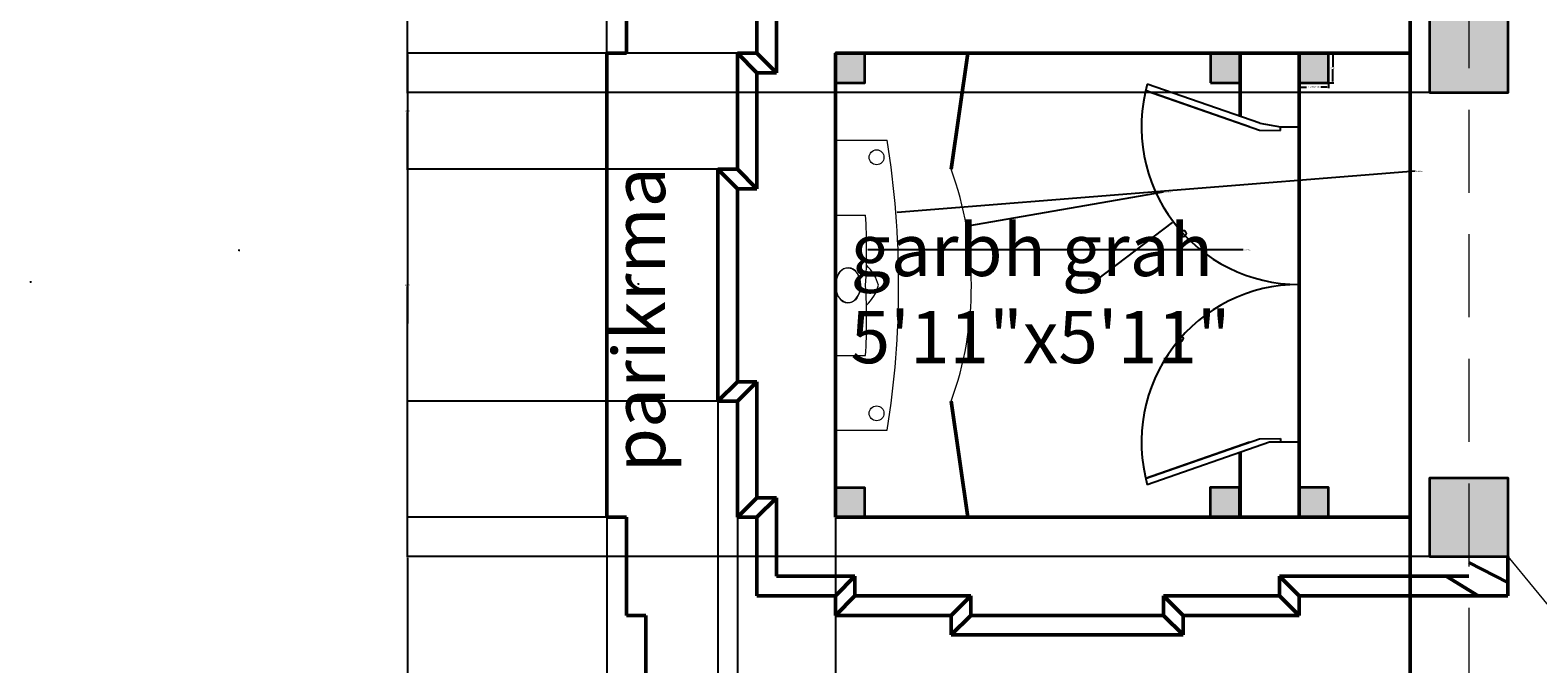
# Model space of a CAD drawing. Units: inches. Extents: x 386 to 107067, y -7 to 96314.
# Tile 4 of 10: x 535 to 766, y 1024 to 1121. Entities that reach past the tile are written whole.
import ezdxf

# ---------------------------------------------------------------- set-up
doc = ezdxf.new("R2010")
doc.units = ezdxf.units.IN
doc.linetypes.add('DASHED', pattern=[19.05, 12.7, -6.35])
for name, color, linetype, lineweight in [('A-ANNO-DIMS', 2, 'Continuous', 18), ('A-AREA-IDEN', 3, 'Continuous', 18), ('A-COLS', 1, 'Continuous', 35), ('A-DOOR', 4, 'Continuous', 25), ('A-FLOR-FIXT', 8, 'Continuous', 18), ('A-FLOR-OVHD', 8, 'DASHED', 18), ('A-WALL', 7, 'Continuous', 50)]:
    doc.layers.add(name, color=color, linetype=linetype, lineweight=lineweight)
doc.styles.get("Standard").update_dxf_attribs({"font": 'arial.ttf'})
doc.dimstyles.get("Standard").update_dxf_attribs({"dimtxt": 0.18, "dimasz": 0.18, "dimexe": 0.18, "dimexo": 0.0625, "dimgap": 0.09, "dimtad": 0, "dimtih": 1, "dimtoh": 1, "dimdec": 4, "dimzin": 0, "dimdsep": 46, "dimtxsty": 'Standard', "dimcen": 0.09, "dimadec": 0, "dimazin": 0, "dimtfac": 1, "dimtdec": 4, "dimtofl": 0, "dimtmove": 0, "dimatfit": 3, "dimfxl": 1, "dimtolj": 1, "dimtzin": 0, "dimarcsym": 0})

# ---------------------------------------------------------------- blocks, each defined once
blk = doc.blocks.new('COL-300')
h = blk.add_hatch(color=256)
h.dxf.hatch_style = 1
h.paths.add_polyline_path([(761.03, 1172.09), (749.03, 1172.09), (749.03, 1160.09), (761.03, 1160.09)])
blk.add_lwpolyline([(749.03, 1160.09), (761.03, 1160.09), (761.03, 1172.09), (749.03, 1172.09)], close=True)
blk = doc.blocks.new('COL-115')
h = blk.add_hatch(color=256)
h.dxf.hatch_style = 1
h.paths.add_polyline_path([(733.53, 1117.59), (729.03, 1117.59), (729.03, 1113.09), (733.53, 1113.09)])
blk.add_lwpolyline([(729.03, 1113.09), (733.53, 1113.09), (733.53, 1117.59), (729.03, 1117.59)], close=True)
blk = doc.blocks.new('*D6')
at = {"layer": 'A-ANNO-DIMS', "color": 0, "lineweight": -2, "transparency": 16777216}
for p, q in [((729.03, 1113.03), (729.03, 1112.24)), ((733.53, 1113.03), (733.53, 1112.24)), ((729.21, 1112.42), (730.18, 1112.42)), ((733.35, 1112.42), (732.37, 1112.42))]:
    blk.add_line(p, q, dxfattribs=at)
at = {"layer": 'A-ANNO-DIMS', "color": 0, "transparency": 16777216}
for points in [[(729.21, 1112.45), (729.21, 1112.39), (729.03, 1112.42)], [(733.35, 1112.45), (733.35, 1112.39), (733.53, 1112.42)]]:
    blk.add_solid(points, dxfattribs=at)
at = {"layer": 'Defpoints', "color": 0, "transparency": 16777216}
for p in [(729.03, 1113.09), (733.53, 1113.09), (733.53, 1112.42)]:
    blk.add_point(p, dxfattribs=at)
at = {"layer": 'A-ANNO-DIMS', "color": 0, "transparency": 16777216, "insert": (731.28, 1112.42), "char_height": 0.18, "attachment_point": 5}
blk.add_mtext('\\A1;PILASTER 5 TYP.', dxfattribs=at)
blk = doc.blocks.new('*D7')
at = {"layer": 'A-ANNO-DIMS', "color": 0, "lineweight": -2, "transparency": 16777216}
for p, q in [((733.59, 1117.59), (734.38, 1117.59)), ((734.2, 1117.41), (734.2, 1115.52)), ((734.2, 1113.27), (734.2, 1115.16)), ((733.59, 1113.09), (734.38, 1113.09))]:
    blk.add_line(p, q, dxfattribs=at)
at = {"layer": 'A-ANNO-DIMS', "color": 0, "transparency": 16777216}
for points in [[(734.17, 1117.41), (734.23, 1117.41), (734.2, 1117.59)], [(734.17, 1113.27), (734.23, 1113.27), (734.2, 1113.09)]]:
    blk.add_solid(points, dxfattribs=at)
at = {"layer": 'Defpoints', "color": 0, "transparency": 16777216}
for p in [(733.53, 1117.59), (734.2, 1117.59), (733.53, 1113.09)]:
    blk.add_point(p, dxfattribs=at)
at = {"layer": 'A-ANNO-DIMS', "color": 0, "transparency": 16777216, "insert": (734.2, 1115.34), "char_height": 0.18, "attachment_point": 5}
blk.add_mtext('\\A1;5 TYP.', dxfattribs=at)
blk = doc.blocks.new('*D8')
at = {"layer": 'A-ANNO-DIMS', "color": 0, "lineweight": -2, "transparency": 16777216}
for p, q in [((623.03, 1046.53), (623.03, 872.22)), ((1169.03, 1014.03), (1169.03, 872.22)), ((623.21, 872.4), (895.74, 872.4)), ((1168.85, 872.4), (896.31, 872.4))]:
    blk.add_line(p, q, dxfattribs=at)
at = {"layer": 'A-ANNO-DIMS', "color": 0, "transparency": 16777216}
for points in [[(623.21, 872.43), (623.21, 872.37), (623.03, 872.4)], [(1168.85, 872.43), (1168.85, 872.37), (1169.03, 872.4)]]:
    blk.add_solid(points, dxfattribs=at)
at = {"layer": 'Defpoints', "color": 0, "transparency": 16777216}
for p in [(623.03, 1046.59), (1169.03, 1014.09), (1169.03, 872.4)]:
    blk.add_point(p, dxfattribs=at)
at = {"layer": 'A-ANNO-DIMS', "color": 0, "transparency": 16777216, "insert": (896.03, 872.4), "char_height": 0.18, "attachment_point": 5}
blk.add_mtext('\\A1;546', dxfattribs=at)
blk = doc.blocks.new('*D9')
at = {"layer": 'A-ANNO-DIMS', "color": 0, "lineweight": -2, "transparency": 16777216}
for p, q in [((623.03, 1117.65), (623.03, 1270.77)), ((623.21, 1270.59), (675.74, 1270.59)), ((728.85, 1270.59), (676.31, 1270.59)), ((729.03, 1152.65), (729.03, 1270.77))]:
    blk.add_line(p, q, dxfattribs=at)
at = {"layer": 'A-ANNO-DIMS', "color": 0, "transparency": 16777216}
for points in [[(623.21, 1270.62), (623.21, 1270.56), (623.03, 1270.59)], [(728.85, 1270.62), (728.85, 1270.56), (729.03, 1270.59)]]:
    blk.add_solid(points, dxfattribs=at)
at = {"layer": 'Defpoints', "color": 0, "transparency": 16777216}
for p in [(729.03, 1270.59), (729.03, 1152.59), (623.03, 1117.59)]:
    blk.add_point(p, dxfattribs=at)
at = {"layer": 'A-ANNO-DIMS', "color": 0, "transparency": 16777216, "insert": (676.03, 1270.59), "char_height": 0.18, "attachment_point": 5}
blk.add_mtext('\\A1;106', dxfattribs=at)
blk = doc.blocks.new('*D32')
at = {"layer": 'A-ANNO-DIMS', "color": 0, "lineweight": -2, "transparency": 16777216}
for p, q in [((748.96, 1040.59), (592.35, 1040.59)), ((592.53, 1040.41), (592.53, 1016.52)), ((592.53, 992.27), (592.53, 1016.16)), ((748.96, 992.09), (592.35, 992.09))]:
    blk.add_line(p, q, dxfattribs=at)
at = {"layer": 'A-ANNO-DIMS', "color": 0, "transparency": 16777216}
for points in [[(592.5, 1040.41), (592.56, 1040.41), (592.53, 1040.59)], [(592.5, 992.27), (592.56, 992.27), (592.53, 992.09)]]:
    blk.add_solid(points, dxfattribs=at)
at = {"layer": 'Defpoints', "color": 0, "transparency": 16777216}
for p in [(592.53, 1040.59), (749.03, 1040.59), (749.03, 992.09)]:
    blk.add_point(p, dxfattribs=at)
at = {"layer": 'A-ANNO-DIMS', "color": 0, "transparency": 16777216, "insert": (592.53, 1016.34), "char_height": 0.18, "attachment_point": 5}
blk.add_mtext('\\A1;48.5', dxfattribs=at)
blk = doc.blocks.new('*D33')
at = {"layer": 'A-ANNO-DIMS', "color": 0, "lineweight": -2, "transparency": 16777216}
for p, q in [((748.96, 1111.59), (592.35, 1111.59)), ((592.53, 1111.41), (592.53, 1076.27)), ((592.53, 1040.77), (592.53, 1075.91)), ((748.96, 1040.59), (592.35, 1040.59))]:
    blk.add_line(p, q, dxfattribs=at)
at = {"layer": 'A-ANNO-DIMS', "color": 0, "transparency": 16777216}
for points in [[(592.5, 1111.41), (592.56, 1111.41), (592.53, 1111.59)], [(592.5, 1040.77), (592.56, 1040.77), (592.53, 1040.59)]]:
    blk.add_solid(points, dxfattribs=at)
at = {"layer": 'Defpoints', "color": 0, "transparency": 16777216}
for p in [(592.53, 1111.59), (749.03, 1111.59), (749.03, 1040.59)]:
    blk.add_point(p, dxfattribs=at)
at = {"layer": 'A-ANNO-DIMS', "color": 0, "transparency": 16777216, "insert": (592.53, 1076.09), "char_height": 0.18, "attachment_point": 5}
blk.add_mtext('\\A1;71', dxfattribs=at)
blk = doc.blocks.new('*D34')
at = {"layer": 'A-ANNO-DIMS', "color": 0, "lineweight": -2, "transparency": 16777216}
for p, q in [((748.96, 1160.09), (592.35, 1160.09)), ((592.53, 1159.91), (592.53, 1136.02)), ((592.53, 1111.77), (592.53, 1135.66)), ((748.96, 1111.59), (592.35, 1111.59))]:
    blk.add_line(p, q, dxfattribs=at)
at = {"layer": 'A-ANNO-DIMS', "color": 0, "transparency": 16777216}
for points in [[(592.5, 1159.91), (592.56, 1159.91), (592.53, 1160.09)], [(592.5, 1111.77), (592.56, 1111.77), (592.53, 1111.59)]]:
    blk.add_solid(points, dxfattribs=at)
at = {"layer": 'Defpoints', "color": 0, "transparency": 16777216}
for p in [(592.53, 1160.09), (749.03, 1160.09), (749.03, 1111.59)]:
    blk.add_point(p, dxfattribs=at)
at = {"layer": 'A-ANNO-DIMS', "color": 0, "transparency": 16777216, "insert": (592.53, 1135.84), "char_height": 0.18, "attachment_point": 5}
blk.add_mtext('\\A1;48.5', dxfattribs=at)
blk = doc.blocks.new('*D36')
at = {"layer": 'A-ANNO-DIMS', "color": 0, "lineweight": -2, "transparency": 16777216}
for p, q in [((623.03, 1117.65), (623.03, 1270.77)), ((623.21, 1270.59), (624.38, 1270.59)), ((625.85, 1270.59), (624.67, 1270.59)), ((626.03, 1129.65), (626.03, 1270.77))]:
    blk.add_line(p, q, dxfattribs=at)
at = {"layer": 'A-ANNO-DIMS', "color": 0, "transparency": 16777216}
for points in [[(623.21, 1270.62), (623.21, 1270.56), (623.03, 1270.59)], [(625.85, 1270.62), (625.85, 1270.56), (626.03, 1270.59)]]:
    blk.add_solid(points, dxfattribs=at)
at = {"layer": 'Defpoints', "color": 0, "transparency": 16777216}
for p in [(626.03, 1270.59), (626.03, 1129.59), (623.03, 1117.59)]:
    blk.add_point(p, dxfattribs=at)
at = {"layer": 'A-ANNO-DIMS', "color": 0, "transparency": 16777216, "insert": (624.53, 1270.59), "char_height": 0.18, "attachment_point": 5}
blk.add_mtext('\\A1;3', dxfattribs=at)
blk = doc.blocks.new('*D44')
at = {"layer": 'A-ANNO-DIMS', "color": 0, "lineweight": -2, "transparency": 16777216}
for p, q in [((640.03, 1064.28), (640.03, 872.22)), ((643.03, 1064.28), (643.03, 872.22)), ((640.21, 872.4), (641.38, 872.4)), ((642.85, 872.4), (641.67, 872.4))]:
    blk.add_line(p, q, dxfattribs=at)
at = {"layer": 'A-ANNO-DIMS', "color": 0, "transparency": 16777216}
for points in [[(640.21, 872.43), (640.21, 872.37), (640.03, 872.4)], [(642.85, 872.43), (642.85, 872.37), (643.03, 872.4)]]:
    blk.add_solid(points, dxfattribs=at)
at = {"layer": 'Defpoints', "color": 0, "transparency": 16777216}
for p in [(640.03, 1064.34), (643.03, 1064.34), (643.03, 872.4)]:
    blk.add_point(p, dxfattribs=at)
at = {"layer": 'A-ANNO-DIMS', "color": 0, "transparency": 16777216, "insert": (641.53, 872.4), "char_height": 0.18, "attachment_point": 5}
blk.add_mtext('\\A1;3', dxfattribs=at)
blk = doc.blocks.new('*D45')
at = {"layer": 'A-ANNO-DIMS', "color": 0, "lineweight": -2, "transparency": 16777216}
for p, q in [((643.03, 1046.53), (643.03, 872.22)), ((658.03, 1046.53), (658.03, 872.22)), ((643.21, 872.4), (650.31, 872.4)), ((657.85, 872.4), (650.74, 872.4))]:
    blk.add_line(p, q, dxfattribs=at)
at = {"layer": 'A-ANNO-DIMS', "color": 0, "transparency": 16777216}
for points in [[(643.21, 872.43), (643.21, 872.37), (643.03, 872.4)], [(657.85, 872.43), (657.85, 872.37), (658.03, 872.4)]]:
    blk.add_solid(points, dxfattribs=at)
at = {"layer": 'Defpoints', "color": 0, "transparency": 16777216}
for p in [(643.03, 1046.59), (658.03, 1046.59), (658.03, 872.4)]:
    blk.add_point(p, dxfattribs=at)
at = {"layer": 'A-ANNO-DIMS', "color": 0, "transparency": 16777216, "insert": (650.53, 872.4), "char_height": 0.18, "attachment_point": 5}
blk.add_mtext('\\A1;15', dxfattribs=at)
blk = doc.blocks.new('*D46')
at = {"layer": 'A-ANNO-DIMS', "color": 0, "lineweight": -2, "transparency": 16777216}
for p, q in [((622.96, 1117.59), (592.35, 1117.59)), ((592.53, 1117.41), (592.53, 1082.27)), ((592.53, 1046.77), (592.53, 1081.91)), ((622.96, 1046.59), (592.35, 1046.59))]:
    blk.add_line(p, q, dxfattribs=at)
at = {"layer": 'A-ANNO-DIMS', "color": 0, "transparency": 16777216}
for points in [[(592.5, 1117.41), (592.56, 1117.41), (592.53, 1117.59)], [(592.5, 1046.77), (592.56, 1046.77), (592.53, 1046.59)]]:
    blk.add_solid(points, dxfattribs=at)
at = {"layer": 'Defpoints', "color": 0, "transparency": 16777216}
for p in [(592.53, 1117.59), (623.03, 1117.59), (623.03, 1046.59)]:
    blk.add_point(p, dxfattribs=at)
at = {"layer": 'A-ANNO-DIMS', "color": 0, "transparency": 16777216, "insert": (592.53, 1082.09), "char_height": 0.18, "attachment_point": 5}
blk.add_mtext('\\A1;71', dxfattribs=at)
blk = doc.blocks.new('*D47')
at = {"layer": 'A-ANNO-DIMS', "color": 0, "lineweight": -2, "transparency": 16777216}
for p, q in [((625.96, 1129.59), (592.35, 1129.59)), ((592.53, 1129.41), (592.53, 1123.77)), ((592.53, 1117.77), (592.53, 1123.41)), ((625.96, 1117.59), (592.35, 1117.59))]:
    blk.add_line(p, q, dxfattribs=at)
at = {"layer": 'A-ANNO-DIMS', "color": 0, "transparency": 16777216}
for points in [[(592.5, 1129.41), (592.56, 1129.41), (592.53, 1129.59)], [(592.5, 1117.77), (592.56, 1117.77), (592.53, 1117.59)]]:
    blk.add_solid(points, dxfattribs=at)
at = {"layer": 'Defpoints', "color": 0, "transparency": 16777216}
for p in [(592.53, 1129.59), (626.03, 1129.59), (626.03, 1117.59)]:
    blk.add_point(p, dxfattribs=at)
at = {"layer": 'A-ANNO-DIMS', "color": 0, "transparency": 16777216, "insert": (592.53, 1123.59), "char_height": 0.18, "attachment_point": 5}
blk.add_mtext('\\A1;12', dxfattribs=at)
blk = doc.blocks.new('*D49')
at = {"layer": 'A-ANNO-DIMS', "color": 0, "lineweight": -2, "transparency": 16777216}
for p, q in [((639.96, 1099.84), (592.35, 1099.84)), ((592.53, 1099.66), (592.53, 1082.27)), ((592.53, 1064.52), (592.53, 1081.91)), ((639.96, 1064.34), (592.35, 1064.34))]:
    blk.add_line(p, q, dxfattribs=at)
at = {"layer": 'A-ANNO-DIMS', "color": 0, "transparency": 16777216}
for points in [[(592.5, 1099.66), (592.56, 1099.66), (592.53, 1099.84)], [(592.5, 1064.52), (592.56, 1064.52), (592.53, 1064.34)]]:
    blk.add_solid(points, dxfattribs=at)
at = {"layer": 'Defpoints', "color": 0, "transparency": 16777216}
for p in [(592.53, 1099.84), (640.03, 1099.84), (640.03, 1064.34)]:
    blk.add_point(p, dxfattribs=at)
at = {"layer": 'A-ANNO-DIMS', "color": 0, "transparency": 16777216, "insert": (592.53, 1082.09), "char_height": 0.18, "attachment_point": 5}
blk.add_mtext('\\A1;35.496', dxfattribs=at)
blk = doc.blocks.new('*D50')
at = {"layer": 'A-ANNO-DIMS', "color": 0, "lineweight": -2, "transparency": 16777216}
for p, q in [((642.96, 1117.59), (592.35, 1117.59)), ((592.53, 1117.41), (592.53, 1108.9)), ((592.53, 1100.02), (592.53, 1108.53)), ((642.96, 1099.84), (592.35, 1099.84))]:
    blk.add_line(p, q, dxfattribs=at)
at = {"layer": 'A-ANNO-DIMS', "color": 0, "transparency": 16777216}
for points in [[(592.5, 1117.41), (592.56, 1117.41), (592.53, 1117.59)], [(592.5, 1100.02), (592.56, 1100.02), (592.53, 1099.84)]]:
    blk.add_solid(points, dxfattribs=at)
at = {"layer": 'Defpoints', "color": 0, "transparency": 16777216}
for p in [(592.53, 1117.59), (643.03, 1117.59), (643.03, 1099.84)]:
    blk.add_point(p, dxfattribs=at)
at = {"layer": 'A-ANNO-DIMS', "color": 0, "transparency": 16777216, "insert": (592.53, 1108.71), "char_height": 0.18, "attachment_point": 5}
blk.add_mtext('\\A1;17.756', dxfattribs=at)
blk = doc.blocks.new('*D51')
at = {"layer": 'A-ANNO-DIMS', "color": 0, "lineweight": -2, "transparency": 16777216}
for p, q in [((645.96, 1129.59), (592.35, 1129.59)), ((592.53, 1129.41), (592.53, 1123.77)), ((592.53, 1117.77), (592.53, 1123.41)), ((645.96, 1117.59), (592.35, 1117.59))]:
    blk.add_line(p, q, dxfattribs=at)
at = {"layer": 'A-ANNO-DIMS', "color": 0, "transparency": 16777216}
for points in [[(592.5, 1129.41), (592.56, 1129.41), (592.53, 1129.59)], [(592.5, 1117.77), (592.56, 1117.77), (592.53, 1117.59)]]:
    blk.add_solid(points, dxfattribs=at)
at = {"layer": 'Defpoints', "color": 0, "transparency": 16777216}
for p in [(592.53, 1129.59), (646.03, 1129.59), (646.03, 1117.59)]:
    blk.add_point(p, dxfattribs=at)
at = {"layer": 'A-ANNO-DIMS', "color": 0, "transparency": 16777216, "insert": (592.53, 1123.59), "char_height": 0.18, "attachment_point": 5}
blk.add_mtext('\\A1;12', dxfattribs=at)
blk = doc.blocks.new('*D87')
at = {"layer": 'A-ANNO-DIMS', "color": 0, "lineweight": -2, "transparency": 16777216}
for p, q in [((746.79, 1099.54), (667.48, 1093.21)), ((534.73, 1082.63), (534.91, 1082.63)), ((534.82, 1082.54), (534.82, 1082.72))]:
    blk.add_line(p, q, dxfattribs=at)
at = {"layer": 'A-ANNO-DIMS', "color": 0, "transparency": 16777216}
blk.add_solid([(667.48, 1093.24), (667.48, 1093.18), (667.3, 1093.2)], dxfattribs=at)
at = {"layer": 'Defpoints', "color": 0, "transparency": 16777216}
for p in [(667.3, 1093.2), (534.82, 1082.63)]:
    blk.add_point(p, dxfattribs=at)
at = {"layer": 'A-ANNO-DIMS', "color": 0, "transparency": 16777216, "insert": (747.46, 1099.54), "char_height": 0.18, "attachment_point": 5}
blk.add_mtext('\\A1;2X R132.9', dxfattribs=at)
blk = doc.blocks.new('*D88')
at = {"layer": 'A-ANNO-DIMS', "color": 0, "lineweight": -2, "transparency": 16777216}
for p, q in [((566.66, 1087.46), (566.84, 1087.46)), ((566.75, 1087.37), (566.75, 1087.55)), ((720.45, 1087.53), (662.99, 1087.5))]:
    blk.add_line(p, q, dxfattribs=at)
at = {"layer": 'A-ANNO-DIMS', "color": 0, "transparency": 16777216}
blk.add_solid([(662.99, 1087.53), (662.99, 1087.47), (662.81, 1087.5)], dxfattribs=at)
at = {"layer": 'Defpoints', "color": 0, "transparency": 16777216}
for p in [(566.75, 1087.46), (662.81, 1087.5)]:
    blk.add_point(p, dxfattribs=at)
at = {"layer": 'A-ANNO-DIMS', "color": 0, "transparency": 16777216, "insert": (721.13, 1087.53), "char_height": 0.18, "attachment_point": 5}
blk.add_mtext('\\A1;2X R96.07', dxfattribs=at)
blk = doc.blocks.new('*D89')
at = {"layer": 'A-ANNO-DIMS', "color": 0, "lineweight": -2, "transparency": 16777216}
for p, q in [((708.22, 1096.35), (678.27, 1091.13)), ((627.8, 1082.34), (627.98, 1082.34)), ((627.89, 1082.25), (627.89, 1082.43))]:
    blk.add_line(p, q, dxfattribs=at)
at = {"layer": 'A-ANNO-DIMS', "color": 0, "transparency": 16777216}
blk.add_solid([(678.27, 1091.16), (678.28, 1091.1), (678.09, 1091.1)], dxfattribs=at)
at = {"layer": 'Defpoints', "color": 0, "transparency": 16777216}
for p in [(678.09, 1091.1), (627.89, 1082.34)]:
    blk.add_point(p, dxfattribs=at)
at = {"layer": 'A-ANNO-DIMS', "color": 0, "transparency": 16777216, "insert": (708.89, 1096.35), "char_height": 0.18, "attachment_point": 5}
blk.add_mtext('\\A1;2X R50.96', dxfattribs=at)
blk = doc.blocks.new('*D90')
at = {"layer": 'A-ANNO-DIMS', "color": 0, "lineweight": -2, "transparency": 16777216}
for p, q in [((728.94, 1106.36), (729.12, 1106.36)), ((729.03, 1106.27), (729.03, 1106.45)), ((698.24, 1083.05), (709.64, 1091.68)), ((698.06, 1083.05), (698.24, 1083.05))]:
    blk.add_line(p, q, dxfattribs=at)
at = {"layer": 'A-ANNO-DIMS', "color": 0, "transparency": 16777216}
blk.add_solid([(709.62, 1091.7), (709.66, 1091.66), (709.79, 1091.79)], dxfattribs=at)
at = {"layer": 'Defpoints', "color": 0, "transparency": 16777216}
for p in [(729.03, 1106.36), (709.79, 1091.79)]:
    blk.add_point(p, dxfattribs=at)
at = {"layer": 'A-ANNO-DIMS', "color": 0, "transparency": 16777216, "insert": (697.32, 1083.05), "char_height": 0.18, "attachment_point": 5}
blk.add_mtext('\\A1;2X R24.134', dxfattribs=at)

msp = doc.modelspace()

# ---------------------------------------------------------------- linework, layer by layer
at = {"layer": 'A-DOOR'}
for p, q in [((723.033, 1106.8794), (705.7914, 1112.8881)), ((721.4384, 1106.3593), (705.5411, 1111.9211)), ((705.5411, 1111.9211), (722.9555, 1105.8286)), ((723.033, 1106.8794), (726.1878, 1106.3593)), ((726.1878, 1105.7799), (726.1878, 1106.3593)), ((726.1878, 1106.3593), (729.0252, 1106.3593)), ((729.0252, 1082.0919), (729.0252, 1106.0919)), ((722.9555, 1105.8286), (726.1878, 1105.7799)), ((729.0252, 1082.0919), (729.0252, 1058.0919)), ((705.5411, 1052.5302), (722.9555, 1058.6227)), ((721.4384, 1058.0919), (705.5411, 1052.5302)), ((724.5252, 1058.0919), (705.7914, 1051.5631)), ((722.9555, 1058.6227), (726.1878, 1058.6714)), ((729.0252, 1058.0919), (724.5252, 1058.0919)), ((726.1878, 1058.6714), (726.1878, 1058.0919))]:
    msp.add_line(p, q, dxfattribs=at)
for centre in [(711.2734, 1090.0098), (710.8132, 1073.9273)]:
    msp.add_circle(centre, 0.4856, dxfattribs=at)
for centre, start, end in [((729.0252, 1106.3593), 164.304426, 270), ((729.0252, 1058.0919), 90, 195.695574)]:
    msp.add_arc(centre, 24.1337, start, end, dxfattribs=at)
at = {"layer": 'A-FLOR-FIXT'}
for p, q in [((658.0252, 1104.281), (665.9435, 1104.281)), ((658.0252, 1092.8185), (662.6616, 1092.8185)), ((658.0252, 1082.0919), (658.0672, 1082.0919)), ((658.0252, 1082.0919), (658.0672, 1082.0919)), ((658.0252, 1071.3654), (662.6616, 1071.3654)), ((658.0252, 1059.9029), (665.9435, 1059.9029))]:
    msp.add_line(p, q, dxfattribs=at)
for centre in [(664.3334, 1101.6786), (664.3334, 1062.5053)]:
    msp.add_circle(centre, 1.1388, dxfattribs=at)
for centre, radius, start, end in [((534.8198, 1082.626), 132.8998, 359.769735, 9.377681), ((627.8894, 1082.3399), 50.9625, 359.721203, 20.08597), ((566.7461, 1087.4552), 96.0654, 356.799556, 3.200444), ((658.6286, 1080.5448), 6.2008, 14.448353, 47.92565), ((566.7461, 1076.7287), 96.0654, 356.799556, 3.200444), ((658.6286, 1083.6391), 6.2008, 312.07435, 345.551647), ((534.8198, 1081.5578), 132.8998, 350.622319, 0.230265), ((627.8894, 1081.844), 50.9625, 339.91403, 0.278797)]:
    msp.add_arc(centre, radius, start, end, dxfattribs=at)
msp.add_ellipse((659.9752, 1082.0919), major_axis=(0.0657, -2.6907), ratio=0.70882274, dxfattribs=at)
at = {"layer": 'A-FLOR-FIXT', "extrusion": (0, 0, -1)}
msp.add_ellipse((659.9752, 1082.0919), major_axis=(0.0657, 2.6907), ratio=0.70882274, dxfattribs=at)
at = {"layer": 'A-FLOR-OVHD'}
msp.add_line((761.0252, 1040.5919), (791.0252, 1004.0919), dxfattribs=at)
msp.add_lwpolyline([(755.0252, 998.0919), (923.0252, 998.0919), (923.0252, 1166.0919), (755.0252, 1166.0919)], close=True, dxfattribs=at)
at = {"layer": 'A-WALL'}
for p, q in [((626.0252, 1117.5919), (623.0252, 1117.5919)), ((646.0252, 1117.5919), (643.0252, 1117.5919)), ((643.0252, 1117.5919), (646.0252, 1114.5919)), ((646.0252, 1117.5919), (649.0252, 1114.5919)), ((746.0252, 1117.5919), (658.0252, 1117.5919)), ((675.7522, 1099.8419), (678.3295, 1117.5919)), ((720.0252, 1117.5919), (720.0252, 1107.9276)), ((729.0252, 1117.5919), (729.0252, 1046.5919)), ((649.0252, 1114.5919), (646.0252, 1114.5919)), ((640.0252, 1099.8359), (643.0252, 1099.8359)), ((640.0252, 1099.8359), (643.0252, 1096.8359)), ((643.0252, 1099.8359), (646.0252, 1096.8359)), ((643.0252, 1096.8359), (646.0252, 1096.8359)), ((640.0252, 1064.3399), (643.0252, 1067.3399)), ((643.0252, 1067.3399), (646.0252, 1067.3399)), ((646.0252, 1067.3399), (643.0252, 1064.3399)), ((640.0252, 1064.3399), (643.0252, 1064.3399)), ((675.7522, 1064.3419), (678.3295, 1046.5919)), ((720.0252, 1056.5237), (720.0252, 1046.5919)), ((643.0252, 1046.5919), (646.0252, 1049.5919)), ((649.0252, 1049.5919), (646.0252, 1049.5919)), ((646.0252, 1046.5919), (649.0252, 1049.5919)), ((626.0252, 1046.5919), (623.0252, 1046.5919)), ((626.0252, 1031.5919), (626.0252, 1046.5919)), ((646.0252, 1046.5919), (643.0252, 1046.5919)), ((746.0252, 1046.5919), (658.0252, 1046.5919)), ((761.0252, 1036.6231), (755.0252, 1039.7036)), ((761.0252, 1034.5919), (761.0252, 1040.5919)), ((661.0252, 1037.5919), (649.0252, 1037.5919)), ((658.0252, 1034.5919), (661.0252, 1037.5919)), ((746.0252, 1037.5919), (726.0252, 1037.5919)), ((726.0252, 1034.5919), (726.0252, 1037.5919)), ((726.0252, 1037.5919), (729.0252, 1034.5919)), ((746.0252, 1037.5919), (755.0252, 1037.5919)), ((756.4697, 1034.5919), (751.5774, 1037.5919)), ((658.0252, 1034.5919), (646.0252, 1034.5919)), ((658.0252, 1031.5919), (661.0252, 1034.5919)), ((678.7732, 1034.5919), (661.0252, 1034.5919)), ((675.7732, 1031.5919), (678.7732, 1034.5919)), ((678.7732, 1034.5919), (678.7732, 1031.5919)), ((708.2692, 1034.5919), (708.2692, 1031.5919)), ((726.0252, 1034.5919), (708.2692, 1034.5919)), ((708.2692, 1034.5919), (711.2692, 1031.5919)), ((726.0252, 1034.5919), (729.0252, 1031.5919)), ((746.0252, 1034.5919), (729.0252, 1034.5919)), ((729.0252, 1031.5919), (729.0252, 1034.5919)), ((746.0252, 1034.5919), (761.0252, 1034.5919)), ((629.0252, 1031.5919), (626.0252, 1031.5919)), ((629.0252, 1031.5919), (629.0252, 1017.5919)), ((675.7732, 1031.5919), (658.0252, 1031.5919)), ((675.7732, 1031.5919), (675.7732, 1028.5919)), ((675.7732, 1028.5919), (678.7732, 1031.5919)), ((708.2692, 1031.5919), (678.7732, 1031.5919)), ((708.2692, 1031.5919), (711.2692, 1028.5919)), ((729.0252, 1031.5919), (711.2692, 1031.5919)), ((711.2692, 1031.5919), (711.2692, 1028.5919)), ((711.2692, 1028.5919), (675.7732, 1028.5919))]:
    msp.add_line(p, q, dxfattribs=at)
for points in [[(788.0252, 1175.0919), (746.0252, 1175.0919), (746.0252, 989.0919), (788.0252, 989.0919)], [(626.0252, 1129.5919), (626.0252, 1117.5919)], [(646.0252, 1129.5919), (646.0252, 1117.5919)], [(649.0252, 1126.5919), (649.0252, 1114.5919)], [(623.0252, 1117.5919), (623.0252, 1046.5919)], [(643.0252, 1117.5919), (643.0252, 1099.8359)], [(658.0252, 1117.5919), (658.0252, 1046.5919)], [(646.0252, 1114.5919), (646.0252, 1096.8359)], [(640.0252, 1099.8359), (640.0252, 1064.3399)], [(643.0252, 1096.8359), (643.0252, 1067.3399)], [(646.0252, 1067.3399), (646.0252, 1049.5919)], [(643.0252, 1064.3399), (643.0252, 1046.5919)], [(649.0252, 1049.5919), (649.0252, 1037.5919)], [(646.0252, 1046.5919), (646.0252, 1034.5919)], [(661.0252, 1037.5919), (661.0252, 1034.5919)], [(658.0252, 1034.5919), (658.0252, 1031.5919)]]:
    msp.add_lwpolyline(points, dxfattribs=at)

# ---------------------------------------------------------------- block references
at = {"layer": 'A-COLS'}
for name, p in [('COL-300', (0, -48.5)), ('COL-115', (-71, 0)), ('COL-115', (-13.5486, 0)), ('COL-115', (0, 0)), ('COL-115', (-71, -66.4683)), ('COL-115', (-13.6198, -66.4567)), ('COL-115', (0, -66.4567)), ('COL-300', (0, -119.5))]:
    msp.add_blockref(name, p, dxfattribs=at)

# ---------------------------------------------------------------- texts
at = {"layer": 'A-AREA-IDEN', "insert": (623.9568, 1053.4966), "char_height": 8, "attachment_point": 1, "rotation": 90}
msp.add_mtext_dynamic_manual_height_columns('parikrma', width=177.910198, gutter_width=12.5, heights=[0], dxfattribs=at)
at = {"layer": 'A-AREA-IDEN', "insert": (660.3607, 1091.5069), "char_height": 8, "attachment_point": 1}
msp.add_mtext_dynamic_manual_height_columns('garbh grah\\P5\'11"x5\'11"', width=177.910198, gutter_width=12.5, heights=[0], dxfattribs=at)

# ---------------------------------------------------------------- dimensions: what is measured, and where the dimension line sits
at = {"layer": 'A-ANNO-DIMS'}
for base, p1, p2, picture, middle in [((729.0252, 1270.5919), (623.0252, 1117.5919), (729.0252, 1152.5919), '*D9', (676.0252, 1270.5919)), ((626.0252, 1270.5919), (623.0252, 1117.5919), (626.0252, 1129.5919), '*D36', (624.5252, 1270.5919)), ((643.0252, 872.3951), (640.0252, 1064.3399), (643.0252, 1064.3399), '*D44', (641.5252, 872.3951)), ((1169.0252, 872.3951), (623.0252, 1046.5919), (1169.0252, 1014.0919), '*D8', (896.0252, 872.3951)), ((658.0252, 872.3951), (643.0252, 1046.5919), (658.0252, 1046.5919), '*D45', (650.5252, 872.3951))]:
    dim = msp.add_linear_dim(base=base, p1=p1, p2=p2, dimstyle='Standard', override={"dimdec": 0, "dimlfac": 1, "dimrnd": 0, "dimzin": 0, "dimdsep": 46, "dimlunit": 2}, dxfattribs=at)
    dim.commit()
    dim.dimension.update_dxf_attribs({"geometry": picture, "text_midpoint": middle})
for base, p1, p2, override, picture, middle in [((592.5252, 1160.0919), (749.0252, 1111.5919), (749.0252, 1160.0919), {"dimdec": 1, "dimlfac": 1, "dimrnd": 0, "dimzin": 0, "dimdsep": 46, "dimlunit": 2}, '*D34', (592.5252, 1135.8419)), ((592.5252, 1129.5919), (626.0252, 1117.5919), (626.0252, 1129.5919), {"dimdec": 0, "dimlfac": 1, "dimrnd": 0, "dimzin": 0, "dimdsep": 46, "dimlunit": 2}, '*D47', (592.5252, 1123.5919)), ((592.5252, 1129.5919), (646.0252, 1117.5919), (646.0252, 1129.5919), {"dimdec": 0, "dimlfac": 1, "dimrnd": 0, "dimzin": 0, "dimdsep": 46, "dimlunit": 2}, '*D51', (592.5252, 1123.5919)), ((592.5252, 1117.5919), (643.0252, 1099.8359), (643.0252, 1117.5919), {"dimdec": 3, "dimlfac": 1, "dimrnd": 0, "dimzin": 0, "dimdsep": 46, "dimlunit": 2}, '*D50', (592.5252, 1108.7139)), ((592.5252, 1117.5919), (623.0252, 1046.5919), (623.0252, 1117.5919), {"dimdec": 0, "dimlfac": 1, "dimrnd": 0, "dimzin": 0, "dimdsep": 46, "dimlunit": 2}, '*D46', (592.5252, 1082.0919)), ((592.5252, 1111.5919), (749.0252, 1040.5919), (749.0252, 1111.5919), {"dimdec": 0, "dimlfac": 1, "dimrnd": 0, "dimzin": 0, "dimdsep": 46, "dimlunit": 2}, '*D33', (592.5252, 1076.0919)), ((592.5252, 1099.8359), (640.0252, 1064.3399), (640.0252, 1099.8359), {"dimdec": 3, "dimlfac": 1, "dimrnd": 0, "dimzin": 0, "dimdsep": 46, "dimlunit": 2}, '*D49', (592.5252, 1082.0879)), ((592.5252, 1040.5919), (749.0252, 992.0919), (749.0252, 1040.5919), {"dimdec": 1, "dimlfac": 1, "dimrnd": 0, "dimzin": 0, "dimdsep": 46, "dimlunit": 2}, '*D32', (592.5252, 1016.3419))]:
    dim = msp.add_linear_dim(base=base, p1=p1, p2=p2, angle=90, dimstyle='Standard', override=override, dxfattribs=at)
    dim.commit()
    dim.dimension.update_dxf_attribs({"geometry": picture, "text_midpoint": middle})
dim = msp.add_linear_dim(base=(734.2001952065, 1117.5919411757), p1=(733.5251952065, 1113.0919411757), p2=(733.5251952065, 1117.5919411757), angle=90, text='<> TYP.', dimstyle='Standard', override={"dimdec": 0, "dimlfac": 1, "dimrnd": 0, "dimzin": 0, "dimdsep": 46, "dimlunit": 2}, dxfattribs=at)
dim.commit()
dim.dimension.update_dxf_attribs({"geometry": '*D7', "text_midpoint": (734.2001952065, 1115.3419411757)})
dim = msp.add_linear_dim(base=(733.5251952065, 1112.4169411757), p1=(729.0251952065, 1113.0919411757), p2=(733.5251952065, 1113.0919411757), text='PILASTER <> TYP.', dimstyle='Standard', override={"dimdec": 0, "dimlfac": 1, "dimrnd": 0, "dimzin": 0, "dimdsep": 46, "dimlunit": 2}, dxfattribs=at)
dim.commit()
dim.dimension.update_dxf_attribs({"geometry": '*D6', "text_midpoint": (731.2751952065, 1112.4169411757)})
for center, mpoint, override, picture, middle in [((729.0252, 1106.3593), (709.7859, 1091.7893), {"dimdec": 3, "dimlfac": 1, "dimrnd": 0, "dimzin": 0, "dimdsep": 46, "dimlunit": 2}, '*D90', (697.318, 1083.0473)), ((534.8198, 1082.626), (667.2983, 1093.1999), {"dimdec": 1, "dimlfac": 1, "dimrnd": 0, "dimzin": 0, "dimdsep": 46, "dimlunit": 2}, '*D87', (746.7855, 1099.5442)), ((627.8894, 1082.3399), (678.0935, 1091.0989), {"dimdec": 2, "dimlfac": 1, "dimrnd": 0, "dimzin": 0, "dimdsep": 46, "dimlunit": 2}, '*D89', (708.216, 1096.3542)), ((566.7461, 1087.4552), (662.8115, 1087.5), {"dimdec": 2, "dimlfac": 1, "dimrnd": 0, "dimzin": 0, "dimdsep": 46, "dimlunit": 2}, '*D88', (720.4507, 1087.5269))]:
    dim = msp.add_radius_dim(center=center, mpoint=mpoint, text='2X <>', dimstyle='Standard', override=override, dxfattribs=at)
    dim.commit()
    dim.dimension.update_dxf_attribs({"geometry": picture, "text_midpoint": middle, "dimtype": 164})

doc.saveas('drawing.dxf')
